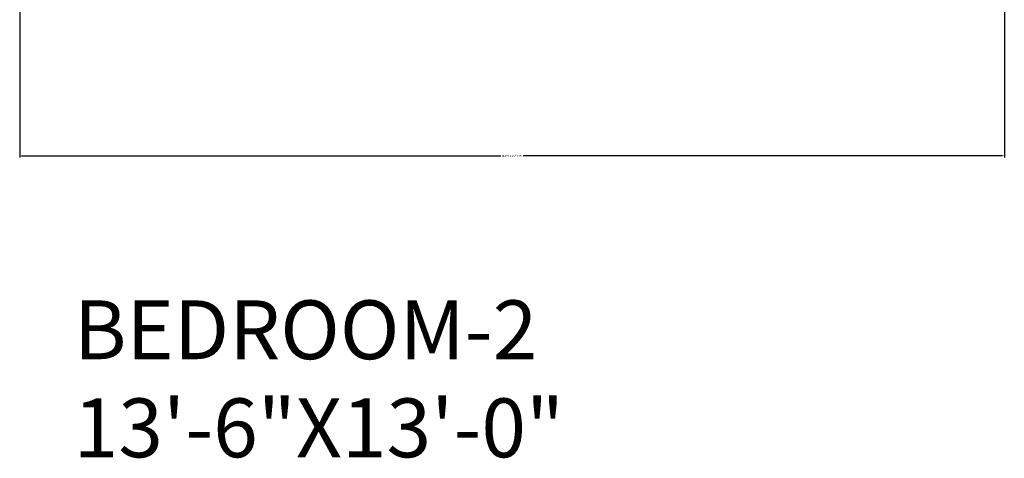
# Model space of a CAD drawing. Units: inches. Extents: x -15 to 423, y -713 to 71.
# Tile 18 of 24: x 262 to 362, y -218 to -173. Entities that reach past the tile are written whole.
import ezdxf

# ---------------------------------------------------------------- set-up
doc = ezdxf.new("R2010")
doc.units = ezdxf.units.IN
doc.header["$MEASUREMENT"] = 0
doc.layers.add('A-ANNO-DIMS', color=2, linetype='Continuous', lineweight=18)
doc.layers.add('A-AREA-IDEN', color=7, linetype='Continuous', lineweight=18)
doc.styles.get("Standard").update_dxf_attribs({"font": 'arial.ttf'})
doc.dimstyles.get("Standard").update_dxf_attribs({"dimtxt": 0.18, "dimasz": 0.18, "dimexe": 0.18, "dimexo": 0.0625, "dimgap": 0.09, "dimtad": 0, "dimtih": 1, "dimtoh": 1, "dimdec": 0, "dimzin": 0, "dimdsep": 46, "dimlunit": 3, "dimtxsty": 'Standard', "dimcen": 0.09, "dimadec": 0, "dimazin": 0, "dimtfac": 1, "dimtdec": 0, "dimtofl": 0, "dimtmove": 0, "dimatfit": 3, "dimfxl": 1, "dimtolj": 1, "dimtzin": 0, "dimarcsym": 0})

# ---------------------------------------------------------------- blocks, each defined once
blk = doc.blocks.new('*D31')
at = {"layer": 'A-ANNO-DIMS', "color": 0, "lineweight": -2, "transparency": 16777216}
for p, q in [((261.64, -171.99), (261.64, -187.15)), ((361.91, -171.99), (361.91, -187.15)), ((261.82, -186.97), (310.63, -186.97)), ((361.73, -186.97), (312.91, -186.97))]:
    blk.add_line(p, q, dxfattribs=at)
at = {"layer": 'A-ANNO-DIMS', "color": 0, "transparency": 16777216}
for points in [[(261.82, -186.94), (261.82, -187), (261.64, -186.97)], [(361.73, -186.94), (361.73, -187), (361.91, -186.97)]]:
    blk.add_solid(points, dxfattribs=at)
at = {"layer": 'Defpoints', "color": 0, "transparency": 16777216}
for p in [(261.64, -171.93), (361.91, -171.93), (361.91, -186.97)]:
    blk.add_point(p, dxfattribs=at)
at = {"layer": 'A-ANNO-DIMS', "color": 0, "transparency": 16777216, "insert": (311.77, -186.97), "char_height": 0.18, "attachment_point": 5}
blk.add_mtext('\\A1;BED 8\'-4 1/2" TYP.', dxfattribs=at)

msp = doc.modelspace()

# ---------------------------------------------------------------- texts
at = {"layer": 'A-AREA-IDEN', "insert": (267.14, -201.71), "char_height": 6, "attachment_point": 1}
msp.add_mtext('BEDROOM-2\\P13\'-6"X13\'-0"', dxfattribs=at)

# ---------------------------------------------------------------- dimensions: what is measured, and where the dimension line sits
at = {"layer": 'A-ANNO-DIMS'}
dim = msp.add_linear_dim(base=(361.91, -186.97), p1=(261.64, -171.93), p2=(361.91, -171.93), text='BED <> TYP.', dimstyle='Standard', override={"dimdec": 1, "dimlfac": 1, "dimrnd": 0, "dimzin": 1, "dimdsep": 46, "dimlunit": 4, "dimfrac": 2}, dxfattribs=at)
dim.commit()
dim.dimension.update_dxf_attribs({"geometry": '*D31', "text_midpoint": (311.77, -186.97)})

doc.saveas('drawing.dxf')
